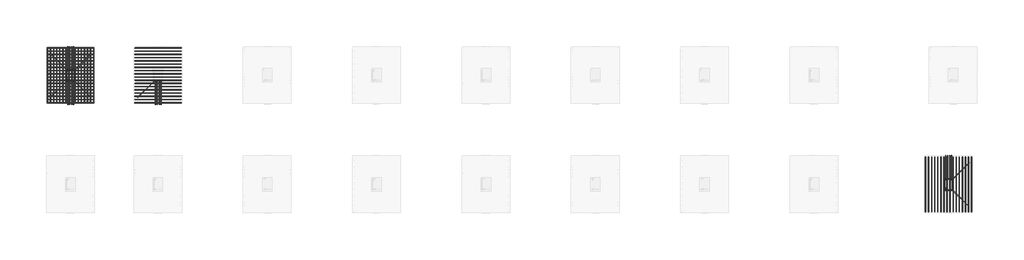
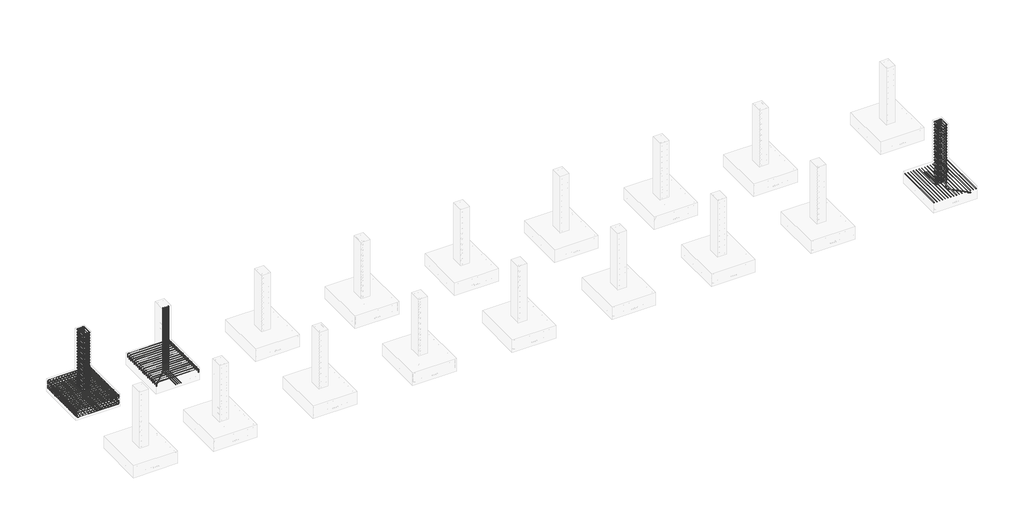
# One storey, part 13 of 33: 19 reinforcing bars.
"""IFC4 building model written with IfcOpenShell, lengths in millimetres."""

from ifc_helpers import new_model, si_unit, point, frame, origin, place, context, project, spatial, polyline, circle_curve, trimmed, segment, composite_curve, source, transform, mapped, element, save
from ifc_brep_helpers import swept_disk

model = new_model("IFC4")

# Units and contexts
model_context = context("Model", 3, world=origin())
ifc_project = project(units=[si_unit("LENGTHUNIT", "METRE", prefix="MILLI")], contexts=[model_context])

# Site, building, storey
site = spatial("IfcSite", under=ifc_project)
building = spatial("IfcBuilding", under=site)
storey = spatial("IfcBuildingStorey", under=building, Elevation=-3000.0)

# Reinforcing bars
placement = place(None, origin())
reinforcing_bar_shape = source(origin(), model_context, "Body", "SolidModel", [
    swept_disk(composite_curve([segment(polyline([(25452.7737106, -4557.7108134, -3122.7084113), (25452.7737106, -2037.7108134, -3122.7084113)]), True, "CONTINUOUS")], self_intersect=False), 6.35),
])
element("IfcReinforcingBar", 1, at=placement, inside=storey, context=model_context, shape_type="MappedRepresentation", body=[
    mapped(reinforcing_bar_shape, transform((0.0, 0.0, 0.0), x_axis=(1.0, 0.0, 0.0), y_axis=(0.0, 1.0, 0.0), z_axis=(0.0, 0.0, 1.0))),
    mapped(reinforcing_bar_shape, transform((140.4866667, 0.0, 0.0), x_axis=(1.0, 0.0, 0.0), y_axis=(0.0, 1.0, 0.0), z_axis=(0.0, 0.0, 1.0))),
    mapped(reinforcing_bar_shape, transform((280.9733333, 0.0, 0.0), x_axis=(1.0, 0.0, 0.0), y_axis=(0.0, 1.0, 0.0), z_axis=(0.0, 0.0, 1.0))),
    mapped(reinforcing_bar_shape, transform((421.46, 0.0, 0.0), x_axis=(1.0, 0.0, 0.0), y_axis=(0.0, 1.0, 0.0), z_axis=(0.0, 0.0, 1.0))),
    mapped(reinforcing_bar_shape, transform((561.9466667, 0.0, 0.0), x_axis=(1.0, 0.0, 0.0), y_axis=(0.0, 1.0, 0.0), z_axis=(0.0, 0.0, 1.0))),
    mapped(reinforcing_bar_shape, transform((702.4333333, 0.0, 0.0), x_axis=(1.0, 0.0, 0.0), y_axis=(0.0, 1.0, 0.0), z_axis=(0.0, 0.0, 1.0))),
    mapped(reinforcing_bar_shape, transform((842.92, 0.0, 0.0), x_axis=(1.0, 0.0, 0.0), y_axis=(0.0, 1.0, 0.0), z_axis=(0.0, 0.0, 1.0))),
    mapped(reinforcing_bar_shape, transform((983.4066667, 0.0, 0.0), x_axis=(1.0, 0.0, 0.0), y_axis=(0.0, 1.0, 0.0), z_axis=(0.0, 0.0, 1.0))),
    mapped(reinforcing_bar_shape, transform((1123.8933333, 0.0, 0.0), x_axis=(1.0, 0.0, 0.0), y_axis=(0.0, 1.0, 0.0), z_axis=(0.0, 0.0, 1.0))),
    mapped(reinforcing_bar_shape, transform((1264.38, 0.0, 0.0), x_axis=(1.0, 0.0, 0.0), y_axis=(0.0, 1.0, 0.0), z_axis=(0.0, 0.0, 1.0))),
    mapped(reinforcing_bar_shape, transform((1404.8666667, 0.0, 0.0), x_axis=(1.0, 0.0, 0.0), y_axis=(0.0, 1.0, 0.0), z_axis=(0.0, 0.0, 1.0))),
    mapped(reinforcing_bar_shape, transform((1545.3533333, 0.0, 0.0), x_axis=(1.0, 0.0, 0.0), y_axis=(0.0, 1.0, 0.0), z_axis=(0.0, 0.0, 1.0))),
    mapped(reinforcing_bar_shape, transform((1685.84, 0.0, 0.0), x_axis=(1.0, 0.0, 0.0), y_axis=(0.0, 1.0, 0.0), z_axis=(0.0, 0.0, 1.0))),
    mapped(reinforcing_bar_shape, transform((1826.3266667, 0.0, 0.0), x_axis=(1.0, 0.0, 0.0), y_axis=(0.0, 1.0, 0.0), z_axis=(0.0, 0.0, 1.0))),
    mapped(reinforcing_bar_shape, transform((1966.8133333, 0.0, 0.0), x_axis=(1.0, 0.0, 0.0), y_axis=(0.0, 1.0, 0.0), z_axis=(0.0, 0.0, 1.0))),
    mapped(reinforcing_bar_shape, transform((2107.3, 0.0, 0.0), x_axis=(1.0, 0.0, 0.0), y_axis=(0.0, 1.0, 0.0), z_axis=(0.0, 0.0, 1.0))),
])
reinforcing_bar_2_shape = source(origin(), model_context, "Body", "SolidModel", [
    swept_disk(composite_curve([segment(polyline([(-10693.4642742, 2955.9391866, -3240.0), (-10693.4642742, 2955.9391866, -3092.7)]), True, "CONTINUOUS"), segment(trimmed(circle_curve(frame((-10647.1142742, 2955.9391866, -3092.7), z_axis=(0.0, 1.0, 0.0), x_axis=(-46.350000000000364, 0.0, 0.0)), 46.35), [point((-10693.4642742, 2955.9391866, -3092.7))], [point((-10647.1142742, 2955.9391866, -3046.35))], True, "CARTESIAN"), True, "CONTINUOUS"), segment(polyline([(-10647.1142742, 2955.9391866, -3046.35), (-8632.5142742, 2955.9391866, -3046.35)]), True, "CONTINUOUS"), segment(trimmed(circle_curve(frame((-8632.5142742, 2955.9391866, -3092.7), z_axis=(0.0, 1.0, 0.0), x_axis=(0.0, 0.0, 46.34999999999991)), 46.35), [point((-8632.5142742, 2955.9391866, -3046.35))], [point((-8586.1642742, 2955.9391866, -3092.7))], True, "CARTESIAN"), True, "CONTINUOUS"), segment(polyline([(-8586.1642742, 2955.9391866, -3092.7), (-8586.1642742, 2955.9391866, -3240.0)]), True, "CONTINUOUS")], self_intersect=False), 6.35),
])
element("IfcReinforcingBar", 2, at=placement, inside=storey, context=model_context, shape_type="MappedRepresentation", body=[
    mapped(reinforcing_bar_2_shape, transform((0.0, 0.0, 0.0), x_axis=(1.0, 0.0, 0.0), y_axis=(0.0, 1.0, 0.0), z_axis=(0.0, 0.0, 1.0))),
    mapped(reinforcing_bar_2_shape, transform((0.0, -147.4882353, 0.0), x_axis=(1.0, 0.0, 0.0), y_axis=(0.0, 1.0, 0.0), z_axis=(0.0, 0.0, 1.0))),
    mapped(reinforcing_bar_2_shape, transform((0.0, -294.9764706, 0.0), x_axis=(1.0, 0.0, 0.0), y_axis=(0.0, 1.0, 0.0), z_axis=(0.0, 0.0, 1.0))),
    mapped(reinforcing_bar_2_shape, transform((0.0, -442.4647059, 0.0), x_axis=(1.0, 0.0, 0.0), y_axis=(0.0, 1.0, 0.0), z_axis=(0.0, 0.0, 1.0))),
    mapped(reinforcing_bar_2_shape, transform((0.0, -589.9529412, 0.0), x_axis=(1.0, 0.0, 0.0), y_axis=(0.0, 1.0, 0.0), z_axis=(0.0, 0.0, 1.0))),
    mapped(reinforcing_bar_2_shape, transform((0.0, -737.4411765, 0.0), x_axis=(1.0, 0.0, 0.0), y_axis=(0.0, 1.0, 0.0), z_axis=(0.0, 0.0, 1.0))),
    mapped(reinforcing_bar_2_shape, transform((0.0, -884.9294118, 0.0), x_axis=(1.0, 0.0, 0.0), y_axis=(0.0, 1.0, 0.0), z_axis=(0.0, 0.0, 1.0))),
    mapped(reinforcing_bar_2_shape, transform((0.0, -1032.4176471, 0.0), x_axis=(1.0, 0.0, 0.0), y_axis=(0.0, 1.0, 0.0), z_axis=(0.0, 0.0, 1.0))),
    mapped(reinforcing_bar_2_shape, transform((0.0, -1179.9058824, 0.0), x_axis=(1.0, 0.0, 0.0), y_axis=(0.0, 1.0, 0.0), z_axis=(0.0, 0.0, 1.0))),
    mapped(reinforcing_bar_2_shape, transform((0.0, -1327.3941176, 0.0), x_axis=(1.0, 0.0, 0.0), y_axis=(0.0, 1.0, 0.0), z_axis=(0.0, 0.0, 1.0))),
    mapped(reinforcing_bar_2_shape, transform((0.0, -1474.8823529, 0.0), x_axis=(1.0, 0.0, 0.0), y_axis=(0.0, 1.0, 0.0), z_axis=(0.0, 0.0, 1.0))),
    mapped(reinforcing_bar_2_shape, transform((0.0, -1622.3705882, 0.0), x_axis=(1.0, 0.0, 0.0), y_axis=(0.0, 1.0, 0.0), z_axis=(0.0, 0.0, 1.0))),
    mapped(reinforcing_bar_2_shape, transform((0.0, -1769.8588235, 0.0), x_axis=(1.0, 0.0, 0.0), y_axis=(0.0, 1.0, 0.0), z_axis=(0.0, 0.0, 1.0))),
    mapped(reinforcing_bar_2_shape, transform((0.0, -1917.3470588, 0.0), x_axis=(1.0, 0.0, 0.0), y_axis=(0.0, 1.0, 0.0), z_axis=(0.0, 0.0, 1.0))),
    mapped(reinforcing_bar_2_shape, transform((0.0, -2064.8352941, 0.0), x_axis=(1.0, 0.0, 0.0), y_axis=(0.0, 1.0, 0.0), z_axis=(0.0, 0.0, 1.0))),
    mapped(reinforcing_bar_2_shape, transform((0.0, -2212.3235294, 0.0), x_axis=(1.0, 0.0, 0.0), y_axis=(0.0, 1.0, 0.0), z_axis=(0.0, 0.0, 1.0))),
    mapped(reinforcing_bar_2_shape, transform((0.0, -2359.8117647, 0.0), x_axis=(1.0, 0.0, 0.0), y_axis=(0.0, 1.0, 0.0), z_axis=(0.0, 0.0, 1.0))),
    mapped(reinforcing_bar_2_shape, transform((0.0, -2507.3, 0.0), x_axis=(1.0, 0.0, 0.0), y_axis=(0.0, 1.0, 0.0), z_axis=(0.0, 0.0, 1.0))),
])
reinforcing_bar_3_shape = source(origin(), model_context, "Body", "SolidModel", [
    swept_disk(composite_curve([segment(polyline([(-14693.4642742, 2955.9391866, -3240.0), (-14693.4642742, 2955.9391866, -3092.7)]), True, "CONTINUOUS"), segment(trimmed(circle_curve(frame((-14647.1142742, 2955.9391866, -3092.7), z_axis=(0.0, 1.0, 0.0), x_axis=(-46.350000000000364, 0.0, 0.0)), 46.35), [point((-14693.4642742, 2955.9391866, -3092.7))], [point((-14647.1142742, 2955.9391866, -3046.35))], True, "CARTESIAN"), True, "CONTINUOUS"), segment(polyline([(-14647.1142742, 2955.9391866, -3046.35), (-12632.5142742, 2955.9391866, -3046.35)]), True, "CONTINUOUS"), segment(trimmed(circle_curve(frame((-12632.5142742, 2955.9391866, -3092.7), z_axis=(0.0, 1.0, 0.0), x_axis=(0.0, 0.0, 46.34999999999991)), 46.35), [point((-12632.5142742, 2955.9391866, -3046.35))], [point((-12586.1642742, 2955.9391866, -3092.7))], True, "CARTESIAN"), True, "CONTINUOUS"), segment(polyline([(-12586.1642742, 2955.9391866, -3092.7), (-12586.1642742, 2955.9391866, -3240.0)]), True, "CONTINUOUS")], self_intersect=False), 6.35),
])
element("IfcReinforcingBar", 3, at=placement, inside=storey, context=model_context, shape_type="MappedRepresentation", body=[
    mapped(reinforcing_bar_3_shape, transform((0.0, 0.0, 0.0), x_axis=(1.0, 0.0, 0.0), y_axis=(0.0, 1.0, 0.0), z_axis=(0.0, 0.0, 1.0))),
    mapped(reinforcing_bar_3_shape, transform((0.0, -147.4882353, 0.0), x_axis=(1.0, 0.0, 0.0), y_axis=(0.0, 1.0, 0.0), z_axis=(0.0, 0.0, 1.0))),
    mapped(reinforcing_bar_3_shape, transform((0.0, -294.9764706, 0.0), x_axis=(1.0, 0.0, 0.0), y_axis=(0.0, 1.0, 0.0), z_axis=(0.0, 0.0, 1.0))),
    mapped(reinforcing_bar_3_shape, transform((0.0, -442.4647059, 0.0), x_axis=(1.0, 0.0, 0.0), y_axis=(0.0, 1.0, 0.0), z_axis=(0.0, 0.0, 1.0))),
    mapped(reinforcing_bar_3_shape, transform((0.0, -589.9529412, 0.0), x_axis=(1.0, 0.0, 0.0), y_axis=(0.0, 1.0, 0.0), z_axis=(0.0, 0.0, 1.0))),
    mapped(reinforcing_bar_3_shape, transform((0.0, -737.4411765, 0.0), x_axis=(1.0, 0.0, 0.0), y_axis=(0.0, 1.0, 0.0), z_axis=(0.0, 0.0, 1.0))),
    mapped(reinforcing_bar_3_shape, transform((0.0, -884.9294118, 0.0), x_axis=(1.0, 0.0, 0.0), y_axis=(0.0, 1.0, 0.0), z_axis=(0.0, 0.0, 1.0))),
    mapped(reinforcing_bar_3_shape, transform((0.0, -1032.4176471, 0.0), x_axis=(1.0, 0.0, 0.0), y_axis=(0.0, 1.0, 0.0), z_axis=(0.0, 0.0, 1.0))),
    mapped(reinforcing_bar_3_shape, transform((0.0, -1179.9058824, 0.0), x_axis=(1.0, 0.0, 0.0), y_axis=(0.0, 1.0, 0.0), z_axis=(0.0, 0.0, 1.0))),
    mapped(reinforcing_bar_3_shape, transform((0.0, -1327.3941176, 0.0), x_axis=(1.0, 0.0, 0.0), y_axis=(0.0, 1.0, 0.0), z_axis=(0.0, 0.0, 1.0))),
    mapped(reinforcing_bar_3_shape, transform((0.0, -1474.8823529, 0.0), x_axis=(1.0, 0.0, 0.0), y_axis=(0.0, 1.0, 0.0), z_axis=(0.0, 0.0, 1.0))),
    mapped(reinforcing_bar_3_shape, transform((0.0, -1622.3705882, 0.0), x_axis=(1.0, 0.0, 0.0), y_axis=(0.0, 1.0, 0.0), z_axis=(0.0, 0.0, 1.0))),
    mapped(reinforcing_bar_3_shape, transform((0.0, -1769.8588235, 0.0), x_axis=(1.0, 0.0, 0.0), y_axis=(0.0, 1.0, 0.0), z_axis=(0.0, 0.0, 1.0))),
    mapped(reinforcing_bar_3_shape, transform((0.0, -1917.3470588, 0.0), x_axis=(1.0, 0.0, 0.0), y_axis=(0.0, 1.0, 0.0), z_axis=(0.0, 0.0, 1.0))),
    mapped(reinforcing_bar_3_shape, transform((0.0, -2064.8352941, 0.0), x_axis=(1.0, 0.0, 0.0), y_axis=(0.0, 1.0, 0.0), z_axis=(0.0, 0.0, 1.0))),
    mapped(reinforcing_bar_3_shape, transform((0.0, -2212.3235294, 0.0), x_axis=(1.0, 0.0, 0.0), y_axis=(0.0, 1.0, 0.0), z_axis=(0.0, 0.0, 1.0))),
    mapped(reinforcing_bar_3_shape, transform((0.0, -2359.8117647, 0.0), x_axis=(1.0, 0.0, 0.0), y_axis=(0.0, 1.0, 0.0), z_axis=(0.0, 0.0, 1.0))),
    mapped(reinforcing_bar_3_shape, transform((0.0, -2507.3, 0.0), x_axis=(1.0, 0.0, 0.0), y_axis=(0.0, 1.0, 0.0), z_axis=(0.0, 0.0, 1.0))),
])
reinforcing_bar_4_shape = source(origin(), model_context, "Body", "SolidModel", [
    swept_disk(composite_curve([segment(polyline([(-12586.1642742, 2955.9391866, -3330.080452), (-12586.1642742, 2955.9391866, -3477.380452)]), True, "CONTINUOUS"), segment(trimmed(circle_curve(frame((-12632.5142742, 2955.9391866, -3477.380452), z_axis=(0.0, 1.0, 0.0), x_axis=(46.350000000000364, 0.0, 0.0)), 46.35), [point((-12586.1642742, 2955.9391866, -3477.380452))], [point((-12632.5142742, 2955.9391866, -3523.730452))], True, "CARTESIAN"), True, "CONTINUOUS"), segment(polyline([(-12632.5142742, 2955.9391866, -3523.730452), (-14647.1142742, 2955.9391866, -3523.730452)]), True, "CONTINUOUS"), segment(trimmed(circle_curve(frame((-14647.1142742, 2955.9391866, -3477.380452), z_axis=(0.0, 1.0, 0.0), x_axis=(0.0, 0.0, -46.34999999999991)), 46.35), [point((-14647.1142742, 2955.9391866, -3523.730452))], [point((-14693.4642742, 2955.9391866, -3477.380452))], True, "CARTESIAN"), True, "CONTINUOUS"), segment(polyline([(-14693.4642742, 2955.9391866, -3477.380452), (-14693.4642742, 2955.9391866, -3330.080452)]), True, "CONTINUOUS")], self_intersect=False), 6.35),
])
element("IfcReinforcingBar", 4, at=placement, inside=storey, context=model_context, shape_type="MappedRepresentation", body=[
    mapped(reinforcing_bar_4_shape, transform((0.0, 0.0, 0.0), x_axis=(1.0, 0.0, 0.0), y_axis=(0.0, 1.0, 0.0), z_axis=(0.0, 0.0, 1.0))),
    mapped(reinforcing_bar_4_shape, transform((0.0, -147.4882353, 0.0), x_axis=(1.0, 0.0, 0.0), y_axis=(0.0, 1.0, 0.0), z_axis=(0.0, 0.0, 1.0))),
    mapped(reinforcing_bar_4_shape, transform((0.0, -294.9764706, 0.0), x_axis=(1.0, 0.0, 0.0), y_axis=(0.0, 1.0, 0.0), z_axis=(0.0, 0.0, 1.0))),
    mapped(reinforcing_bar_4_shape, transform((0.0, -442.4647059, 0.0), x_axis=(1.0, 0.0, 0.0), y_axis=(0.0, 1.0, 0.0), z_axis=(0.0, 0.0, 1.0))),
    mapped(reinforcing_bar_4_shape, transform((0.0, -589.9529412, 0.0), x_axis=(1.0, 0.0, 0.0), y_axis=(0.0, 1.0, 0.0), z_axis=(0.0, 0.0, 1.0))),
    mapped(reinforcing_bar_4_shape, transform((0.0, -737.4411765, 0.0), x_axis=(1.0, 0.0, 0.0), y_axis=(0.0, 1.0, 0.0), z_axis=(0.0, 0.0, 1.0))),
    mapped(reinforcing_bar_4_shape, transform((0.0, -884.9294118, 0.0), x_axis=(1.0, 0.0, 0.0), y_axis=(0.0, 1.0, 0.0), z_axis=(0.0, 0.0, 1.0))),
    mapped(reinforcing_bar_4_shape, transform((0.0, -1032.4176471, 0.0), x_axis=(1.0, 0.0, 0.0), y_axis=(0.0, 1.0, 0.0), z_axis=(0.0, 0.0, 1.0))),
    mapped(reinforcing_bar_4_shape, transform((0.0, -1179.9058824, 0.0), x_axis=(1.0, 0.0, 0.0), y_axis=(0.0, 1.0, 0.0), z_axis=(0.0, 0.0, 1.0))),
    mapped(reinforcing_bar_4_shape, transform((0.0, -1327.3941176, 0.0), x_axis=(1.0, 0.0, 0.0), y_axis=(0.0, 1.0, 0.0), z_axis=(0.0, 0.0, 1.0))),
    mapped(reinforcing_bar_4_shape, transform((0.0, -1474.8823529, 0.0), x_axis=(1.0, 0.0, 0.0), y_axis=(0.0, 1.0, 0.0), z_axis=(0.0, 0.0, 1.0))),
    mapped(reinforcing_bar_4_shape, transform((0.0, -1622.3705882, 0.0), x_axis=(1.0, 0.0, 0.0), y_axis=(0.0, 1.0, 0.0), z_axis=(0.0, 0.0, 1.0))),
    mapped(reinforcing_bar_4_shape, transform((0.0, -1769.8588235, 0.0), x_axis=(1.0, 0.0, 0.0), y_axis=(0.0, 1.0, 0.0), z_axis=(0.0, 0.0, 1.0))),
    mapped(reinforcing_bar_4_shape, transform((0.0, -1917.3470588, 0.0), x_axis=(1.0, 0.0, 0.0), y_axis=(0.0, 1.0, 0.0), z_axis=(0.0, 0.0, 1.0))),
    mapped(reinforcing_bar_4_shape, transform((0.0, -2064.8352941, 0.0), x_axis=(1.0, 0.0, 0.0), y_axis=(0.0, 1.0, 0.0), z_axis=(0.0, 0.0, 1.0))),
    mapped(reinforcing_bar_4_shape, transform((0.0, -2212.3235294, 0.0), x_axis=(1.0, 0.0, 0.0), y_axis=(0.0, 1.0, 0.0), z_axis=(0.0, 0.0, 1.0))),
    mapped(reinforcing_bar_4_shape, transform((0.0, -2359.8117647, 0.0), x_axis=(1.0, 0.0, 0.0), y_axis=(0.0, 1.0, 0.0), z_axis=(0.0, 0.0, 1.0))),
    mapped(reinforcing_bar_4_shape, transform((0.0, -2507.3, 0.0), x_axis=(1.0, 0.0, 0.0), y_axis=(0.0, 1.0, 0.0), z_axis=(0.0, 0.0, 1.0))),
])
reinforcing_bar_5_shape = source(origin(), model_context, "Body", "SolidModel", [
    swept_disk(composite_curve([segment(polyline([(-12586.1642742, 442.2891866, -3447.8614173), (-12586.1642742, 2962.2891866, -3447.8614173)]), True, "CONTINUOUS")], self_intersect=False), 6.35),
])
element("IfcReinforcingBar", 5, at=placement, inside=storey, context=model_context, shape_type="MappedRepresentation", body=[
    mapped(reinforcing_bar_5_shape, transform((0.0, 0.0, 0.0), x_axis=(1.0, 0.0, 0.0), y_axis=(0.0, 1.0, 0.0), z_axis=(0.0, 0.0, 1.0))),
    mapped(reinforcing_bar_5_shape, transform((-140.4866667, 0.0, 0.0), x_axis=(1.0, 0.0, 0.0), y_axis=(0.0, 1.0, 0.0), z_axis=(0.0, 0.0, 1.0))),
    mapped(reinforcing_bar_5_shape, transform((-280.9733333, 0.0, 0.0), x_axis=(1.0, 0.0, 0.0), y_axis=(0.0, 1.0, 0.0), z_axis=(0.0, 0.0, 1.0))),
    mapped(reinforcing_bar_5_shape, transform((-421.46, 0.0, 0.0), x_axis=(1.0, 0.0, 0.0), y_axis=(0.0, 1.0, 0.0), z_axis=(0.0, 0.0, 1.0))),
    mapped(reinforcing_bar_5_shape, transform((-561.9466667, 0.0, 0.0), x_axis=(1.0, 0.0, 0.0), y_axis=(0.0, 1.0, 0.0), z_axis=(0.0, 0.0, 1.0))),
    mapped(reinforcing_bar_5_shape, transform((-702.4333333, 0.0, 0.0), x_axis=(1.0, 0.0, 0.0), y_axis=(0.0, 1.0, 0.0), z_axis=(0.0, 0.0, 1.0))),
    mapped(reinforcing_bar_5_shape, transform((-842.92, 0.0, 0.0), x_axis=(1.0, 0.0, 0.0), y_axis=(0.0, 1.0, 0.0), z_axis=(0.0, 0.0, 1.0))),
    mapped(reinforcing_bar_5_shape, transform((-983.4066667, 0.0, 0.0), x_axis=(1.0, 0.0, 0.0), y_axis=(0.0, 1.0, 0.0), z_axis=(0.0, 0.0, 1.0))),
    mapped(reinforcing_bar_5_shape, transform((-1123.8933333, 0.0, 0.0), x_axis=(1.0, 0.0, 0.0), y_axis=(0.0, 1.0, 0.0), z_axis=(0.0, 0.0, 1.0))),
    mapped(reinforcing_bar_5_shape, transform((-1264.38, 0.0, 0.0), x_axis=(1.0, 0.0, 0.0), y_axis=(0.0, 1.0, 0.0), z_axis=(0.0, 0.0, 1.0))),
    mapped(reinforcing_bar_5_shape, transform((-1404.8666667, 0.0, 0.0), x_axis=(1.0, 0.0, 0.0), y_axis=(0.0, 1.0, 0.0), z_axis=(0.0, 0.0, 1.0))),
    mapped(reinforcing_bar_5_shape, transform((-1545.3533333, 0.0, 0.0), x_axis=(1.0, 0.0, 0.0), y_axis=(0.0, 1.0, 0.0), z_axis=(0.0, 0.0, 1.0))),
    mapped(reinforcing_bar_5_shape, transform((-1685.84, 0.0, 0.0), x_axis=(1.0, 0.0, 0.0), y_axis=(0.0, 1.0, 0.0), z_axis=(0.0, 0.0, 1.0))),
    mapped(reinforcing_bar_5_shape, transform((-1826.3266667, 0.0, 0.0), x_axis=(1.0, 0.0, 0.0), y_axis=(0.0, 1.0, 0.0), z_axis=(0.0, 0.0, 1.0))),
    mapped(reinforcing_bar_5_shape, transform((-1966.8133333, 0.0, 0.0), x_axis=(1.0, 0.0, 0.0), y_axis=(0.0, 1.0, 0.0), z_axis=(0.0, 0.0, 1.0))),
    mapped(reinforcing_bar_5_shape, transform((-2107.3, 0.0, 0.0), x_axis=(1.0, 0.0, 0.0), y_axis=(0.0, 1.0, 0.0), z_axis=(0.0, 0.0, 1.0))),
])
reinforcing_bar_6_shape = source(origin(), model_context, "Body", "SolidModel", [
    swept_disk(composite_curve([segment(polyline([(-14693.4642742, 442.2891866, -3122.7084113), (-14693.4642742, 2962.2891866, -3122.7084113)]), True, "CONTINUOUS")], self_intersect=False), 6.35),
])
element("IfcReinforcingBar", 6, at=placement, inside=storey, context=model_context, shape_type="MappedRepresentation", body=[
    mapped(reinforcing_bar_6_shape, transform((0.0, 0.0, 0.0), x_axis=(1.0, 0.0, 0.0), y_axis=(0.0, 1.0, 0.0), z_axis=(0.0, 0.0, 1.0))),
    mapped(reinforcing_bar_6_shape, transform((140.4866667, 0.0, 0.0), x_axis=(1.0, 0.0, 0.0), y_axis=(0.0, 1.0, 0.0), z_axis=(0.0, 0.0, 1.0))),
    mapped(reinforcing_bar_6_shape, transform((280.9733333, 0.0, 0.0), x_axis=(1.0, 0.0, 0.0), y_axis=(0.0, 1.0, 0.0), z_axis=(0.0, 0.0, 1.0))),
    mapped(reinforcing_bar_6_shape, transform((421.46, 0.0, 0.0), x_axis=(1.0, 0.0, 0.0), y_axis=(0.0, 1.0, 0.0), z_axis=(0.0, 0.0, 1.0))),
    mapped(reinforcing_bar_6_shape, transform((561.9466667, 0.0, 0.0), x_axis=(1.0, 0.0, 0.0), y_axis=(0.0, 1.0, 0.0), z_axis=(0.0, 0.0, 1.0))),
    mapped(reinforcing_bar_6_shape, transform((702.4333333, 0.0, 0.0), x_axis=(1.0, 0.0, 0.0), y_axis=(0.0, 1.0, 0.0), z_axis=(0.0, 0.0, 1.0))),
    mapped(reinforcing_bar_6_shape, transform((842.92, 0.0, 0.0), x_axis=(1.0, 0.0, 0.0), y_axis=(0.0, 1.0, 0.0), z_axis=(0.0, 0.0, 1.0))),
    mapped(reinforcing_bar_6_shape, transform((983.4066667, 0.0, 0.0), x_axis=(1.0, 0.0, 0.0), y_axis=(0.0, 1.0, 0.0), z_axis=(0.0, 0.0, 1.0))),
    mapped(reinforcing_bar_6_shape, transform((1123.8933333, 0.0, 0.0), x_axis=(1.0, 0.0, 0.0), y_axis=(0.0, 1.0, 0.0), z_axis=(0.0, 0.0, 1.0))),
    mapped(reinforcing_bar_6_shape, transform((1264.38, 0.0, 0.0), x_axis=(1.0, 0.0, 0.0), y_axis=(0.0, 1.0, 0.0), z_axis=(0.0, 0.0, 1.0))),
    mapped(reinforcing_bar_6_shape, transform((1404.8666667, 0.0, 0.0), x_axis=(1.0, 0.0, 0.0), y_axis=(0.0, 1.0, 0.0), z_axis=(0.0, 0.0, 1.0))),
    mapped(reinforcing_bar_6_shape, transform((1545.3533333, 0.0, 0.0), x_axis=(1.0, 0.0, 0.0), y_axis=(0.0, 1.0, 0.0), z_axis=(0.0, 0.0, 1.0))),
    mapped(reinforcing_bar_6_shape, transform((1685.84, 0.0, 0.0), x_axis=(1.0, 0.0, 0.0), y_axis=(0.0, 1.0, 0.0), z_axis=(0.0, 0.0, 1.0))),
    mapped(reinforcing_bar_6_shape, transform((1826.3266667, 0.0, 0.0), x_axis=(1.0, 0.0, 0.0), y_axis=(0.0, 1.0, 0.0), z_axis=(0.0, 0.0, 1.0))),
    mapped(reinforcing_bar_6_shape, transform((1966.8133333, 0.0, 0.0), x_axis=(1.0, 0.0, 0.0), y_axis=(0.0, 1.0, 0.0), z_axis=(0.0, 0.0, 1.0))),
    mapped(reinforcing_bar_6_shape, transform((2107.3, 0.0, 0.0), x_axis=(1.0, 0.0, 0.0), y_axis=(0.0, 1.0, 0.0), z_axis=(0.0, 0.0, 1.0))),
])
reinforcing_bar_7_shape = source(origin(), model_context, "Body", "SolidModel", [
    swept_disk(composite_curve([segment(polyline([(-13753.5385089, 1553.1005472, -2953.65), (-13809.2820718, 1497.3569842, -2953.65)]), True, "CONTINUOUS"), segment(trimmed(circle_curve(frame((-13787.1142742, 1475.1891866, -2953.65), z_axis=(0.0, 0.0, 1.0), x_axis=(-22.167797600000995, 22.167797599999858, 0.0)), 31.35), [point((-13809.2820718, 1497.3569842, -2953.65))], [point((-13787.1142742, 1443.8391866, -2953.65))], True, "CARTESIAN"), True, "CONTINUOUS"), segment(polyline([(-13787.1142742, 1443.8391866, -2953.65), (-13492.5142742, 1443.8391866, -2953.65)]), True, "CONTINUOUS"), segment(trimmed(circle_curve(frame((-13492.5142742, 1475.1891866, -2953.65), z_axis=(0.0, 0.0, 1.0), x_axis=(0.0, -31.350000000000136, 0.0)), 31.35), [point((-13492.5142742, 1443.8391866, -2953.65))], [point((-13461.1642742, 1475.1891866, -2953.65))], True, "CARTESIAN"), True, "CONTINUOUS"), segment(polyline([(-13461.1642742, 1475.1891866, -2953.65), (-13461.1642742, 1929.3891866, -2953.65)]), True, "CONTINUOUS"), segment(trimmed(circle_curve(frame((-13492.4944891, 1929.3891866, -2954.7636125), z_axis=(-0.0355219283344822, 0.0, 0.9993688971583016), x_axis=(31.33021489999919, 0.0, 1.1136124999998174)), 31.35), [point((-13461.1642742, 1929.3891866, -2953.65))], [point((-13492.4944891, 1960.7391866, -2954.7636125))], True, "CARTESIAN"), True, "CONTINUOUS"), segment(polyline([(-13492.4944891, 1960.7391866, -2954.7636125), (-13787.1340593, 1960.7391866, -2965.2363875)]), True, "CONTINUOUS"), segment(trimmed(circle_curve(frame((-13787.1340593, 1929.3891866, -2965.2363875), z_axis=(-0.0355219283344822, 0.0, 0.9993688971583016), x_axis=(0.0, 31.350000000000136, 0.0)), 31.35), [point((-13787.1340593, 1960.7391866, -2965.2363875))], [point((-13818.4642742, 1929.3891866, -2966.35))], True, "CARTESIAN"), True, "CONTINUOUS"), segment(polyline([(-13818.4642742, 1929.3891866, -2966.35), (-13818.4642742, 1475.1891866, -2966.35)]), True, "CONTINUOUS"), segment(trimmed(circle_curve(frame((-13787.1142742, 1475.1891866, -2966.35), z_axis=(0.0, 0.0, 1.0), x_axis=(-31.350000000000364, 0.0, 0.0)), 31.35), [point((-13818.4642742, 1475.1891866, -2966.35))], [point((-13764.9464766, 1453.021389, -2966.35))], True, "CARTESIAN"), True, "CONTINUOUS"), segment(polyline([(-13764.9464766, 1453.021389, -2966.35), (-13709.2029137, 1508.764952, -2966.35)]), True, "CONTINUOUS")], self_intersect=False), 6.35),
])
element("IfcReinforcingBar", 7, at=placement, inside=storey, context=model_context, shape_type="MappedRepresentation", body=[
    mapped(reinforcing_bar_7_shape, transform((0.0, 0.0, 0.0), x_axis=(1.0, 0.0, 0.0), y_axis=(0.0, 1.0, 0.0), z_axis=(0.0, 0.0, 1.0))),
    mapped(reinforcing_bar_7_shape, transform((0.0, 0.0, 145.365), x_axis=(1.0, 0.0, 0.0), y_axis=(0.0, 1.0, 0.0), z_axis=(0.0, 0.0, 1.0))),
    mapped(reinforcing_bar_7_shape, transform((0.0, 0.0, 290.73), x_axis=(1.0, 0.0, 0.0), y_axis=(0.0, 1.0, 0.0), z_axis=(0.0, 0.0, 1.0))),
    mapped(reinforcing_bar_7_shape, transform((0.0, 0.0, 436.095), x_axis=(1.0, 0.0, 0.0), y_axis=(0.0, 1.0, 0.0), z_axis=(0.0, 0.0, 1.0))),
    mapped(reinforcing_bar_7_shape, transform((0.0, 0.0, 581.46), x_axis=(1.0, 0.0, 0.0), y_axis=(0.0, 1.0, 0.0), z_axis=(0.0, 0.0, 1.0))),
    mapped(reinforcing_bar_7_shape, transform((0.0, 0.0, 726.825), x_axis=(1.0, 0.0, 0.0), y_axis=(0.0, 1.0, 0.0), z_axis=(0.0, 0.0, 1.0))),
    mapped(reinforcing_bar_7_shape, transform((0.0, 0.0, 872.19), x_axis=(1.0, 0.0, 0.0), y_axis=(0.0, 1.0, 0.0), z_axis=(0.0, 0.0, 1.0))),
    mapped(reinforcing_bar_7_shape, transform((0.0, 0.0, 1017.555), x_axis=(1.0, 0.0, 0.0), y_axis=(0.0, 1.0, 0.0), z_axis=(0.0, 0.0, 1.0))),
    mapped(reinforcing_bar_7_shape, transform((0.0, 0.0, 1162.92), x_axis=(1.0, 0.0, 0.0), y_axis=(0.0, 1.0, 0.0), z_axis=(0.0, 0.0, 1.0))),
    mapped(reinforcing_bar_7_shape, transform((0.0, 0.0, 1308.285), x_axis=(1.0, 0.0, 0.0), y_axis=(0.0, 1.0, 0.0), z_axis=(0.0, 0.0, 1.0))),
    mapped(reinforcing_bar_7_shape, transform((0.0, 0.0, 1453.65), x_axis=(1.0, 0.0, 0.0), y_axis=(0.0, 1.0, 0.0), z_axis=(0.0, 0.0, 1.0))),
    mapped(reinforcing_bar_7_shape, transform((0.0, 0.0, 1599.015), x_axis=(1.0, 0.0, 0.0), y_axis=(0.0, 1.0, 0.0), z_axis=(0.0, 0.0, 1.0))),
    mapped(reinforcing_bar_7_shape, transform((0.0, 0.0, 1744.38), x_axis=(1.0, 0.0, 0.0), y_axis=(0.0, 1.0, 0.0), z_axis=(0.0, 0.0, 1.0))),
    mapped(reinforcing_bar_7_shape, transform((0.0, 0.0, 1889.745), x_axis=(1.0, 0.0, 0.0), y_axis=(0.0, 1.0, 0.0), z_axis=(0.0, 0.0, 1.0))),
    mapped(reinforcing_bar_7_shape, transform((0.0, 0.0, 2035.11), x_axis=(1.0, 0.0, 0.0), y_axis=(0.0, 1.0, 0.0), z_axis=(0.0, 0.0, 1.0))),
    mapped(reinforcing_bar_7_shape, transform((0.0, 0.0, 2180.475), x_axis=(1.0, 0.0, 0.0), y_axis=(0.0, 1.0, 0.0), z_axis=(0.0, 0.0, 1.0))),
    mapped(reinforcing_bar_7_shape, transform((0.0, 0.0, 2325.84), x_axis=(1.0, 0.0, 0.0), y_axis=(0.0, 1.0, 0.0), z_axis=(0.0, 0.0, 1.0))),
    mapped(reinforcing_bar_7_shape, transform((0.0, 0.0, 2471.205), x_axis=(1.0, 0.0, 0.0), y_axis=(0.0, 1.0, 0.0), z_axis=(0.0, 0.0, 1.0))),
    mapped(reinforcing_bar_7_shape, transform((0.0, 0.0, 2616.57), x_axis=(1.0, 0.0, 0.0), y_axis=(0.0, 1.0, 0.0), z_axis=(0.0, 0.0, 1.0))),
    mapped(reinforcing_bar_7_shape, transform((0.0, 0.0, 2761.935), x_axis=(1.0, 0.0, 0.0), y_axis=(0.0, 1.0, 0.0), z_axis=(0.0, 0.0, 1.0))),
    mapped(reinforcing_bar_7_shape, transform((0.0, 0.0, 2907.3), x_axis=(1.0, 0.0, 0.0), y_axis=(0.0, 1.0, 0.0), z_axis=(0.0, 0.0, 1.0))),
])
element("IfcReinforcingBar", 8, at=placement, inside=storey, context=model_context, shape_type="SolidModel", body=[
    swept_disk(composite_curve([segment(polyline([(-13786.7956786, 1478.3660586, -40.0), (-13786.7956786, 1478.3660586, -3393.65)]), True, "CONTINUOUS"), segment(trimmed(circle_curve(frame((-13819.5700779, 1445.5916593, -3393.65), z_axis=(-0.7071067811865446, 0.7071067811865505, 0.0), x_axis=(32.77439930000037, 32.77439930000014, 0.0)), 46.35), [point((-13786.7956786, 1478.3660586, -3393.65))], [point((-13819.5700779, 1445.5916593, -3440.0))], True, "CARTESIAN"), True, "CONTINUOUS"), segment(polyline([(-13819.5700779, 1445.5916593, -3440.0), (-14564.6131379, 700.5485993, -3440.0)]), True, "CONTINUOUS")], self_intersect=False), 6.35),
])
element("IfcReinforcingBar", 9, at=placement, inside=storey, context=model_context, shape_type="SolidModel", body=[
    swept_disk(composite_curve([segment(polyline([(-13768.8975726, 1908.3142087, -40.0), (-13768.8975726, 1908.3142087, -3361.434517)]), True, "CONTINUOUS"), segment(trimmed(circle_curve(frame((-13801.6719719, 1941.088608, -3361.434517), z_axis=(0.7071067811865539, 0.7071067811865411, 0.0), x_axis=(32.77439929999855, -32.774399299999914, 0.0)), 46.35), [point((-13768.8975726, 1908.3142087, -3361.434517))], [point((-13801.6719719, 1941.088608, -3407.784517))], True, "CARTESIAN"), True, "CONTINUOUS"), segment(polyline([(-13801.6719719, 1941.088608, -3407.784517), (-14564.6131379, 2704.029774, -3407.784517)]), True, "CONTINUOUS")], self_intersect=False), 6.35),
])
element("IfcReinforcingBar", 10, at=placement, inside=storey, context=model_context, shape_type="SolidModel", body=[
    swept_disk(composite_curve([segment(polyline([(-13492.8328699, 1478.3660586, -40.0), (-13492.8328699, 1478.3660586, -3393.65)]), True, "CONTINUOUS"), segment(trimmed(circle_curve(frame((-13460.0584706, 1445.5916593, -3393.65), z_axis=(-0.7071067811865493, -0.7071067811865459, 0.0), x_axis=(-32.77439929999855, 32.77439930000014, 0.0)), 46.35), [point((-13492.8328699, 1478.3660586, -3393.65))], [point((-13460.0584706, 1445.5916593, -3440.0))], True, "CARTESIAN"), True, "CONTINUOUS"), segment(polyline([(-13460.0584706, 1445.5916593, -3440.0), (-12715.0154106, 700.5485993, -3440.0)]), True, "CONTINUOUS")], self_intersect=False), 6.35),
])
element("IfcReinforcingBar", 11, at=placement, inside=storey, context=model_context, shape_type="SolidModel", body=[
    swept_disk(composite_curve([segment(polyline([(-13474.2315783, 1926.2123147, -30.2564663), (-13474.2315783, 1926.2123147, -3383.9064663)]), True, "CONTINUOUS"), segment(trimmed(circle_curve(frame((-13441.457179, 1958.986714, -3383.9064663), z_axis=(0.7071067811865493, -0.7071067811865459, 0.0), x_axis=(-32.77439929999855, -32.774399299999914, 0.0)), 46.35), [point((-13474.2315783, 1926.2123147, -3383.9064663))], [point((-13441.457179, 1958.986714, -3430.2564663))], True, "CARTESIAN"), True, "CONTINUOUS"), segment(polyline([(-13441.457179, 1958.986714, -3430.2564663), (-12696.414119, 2704.029774, -3430.2564663)]), True, "CONTINUOUS")], self_intersect=False), 6.35),
])
reinforcing_bar_8_shape = source(origin(), model_context, "Body", "SolidModel", [
    swept_disk(composite_curve([segment(polyline([(-13763.8841678, 1928.0721866, -40.0), (-13763.8841678, 1928.0721866, -3393.65)]), True, "CONTINUOUS"), segment(trimmed(circle_curve(frame((-13763.8841678, 1974.4221866, -3393.65), z_axis=(1.0, 0.0, 0.0), x_axis=(0.0, -46.350000000000136, 0.0)), 46.35), [point((-13763.8841678, 1928.0721866, -3393.65))], [point((-13763.8841678, 1974.4221866, -3440.0))], True, "CARTESIAN"), True, "CONTINUOUS"), segment(polyline([(-13763.8841678, 1974.4221866, -3440.0), (-13763.8841678, 3028.0721866, -3440.0)]), True, "CONTINUOUS")], self_intersect=False), 6.35),
])
element("IfcReinforcingBar", 12, at=placement, inside=storey, context=model_context, shape_type="MappedRepresentation", body=[
    mapped(reinforcing_bar_8_shape, transform((0.0, 0.0, 0.0), x_axis=(1.0, 0.0, 0.0), y_axis=(0.0, 1.0, 0.0), z_axis=(0.0, 0.0, 1.0))),
    mapped(reinforcing_bar_8_shape, transform((86.8979716, 0.0, 0.0), x_axis=(1.0, 0.0, 0.0), y_axis=(0.0, 1.0, 0.0), z_axis=(0.0, 0.0, 1.0))),
    mapped(reinforcing_bar_8_shape, transform((173.7959432, 0.0, 0.0), x_axis=(1.0, 0.0, 0.0), y_axis=(0.0, 1.0, 0.0), z_axis=(0.0, 0.0, 1.0))),
    mapped(reinforcing_bar_8_shape, transform((260.6939148, 0.0, 0.0), x_axis=(1.0, 0.0, 0.0), y_axis=(0.0, 1.0, 0.0), z_axis=(0.0, 0.0, 1.0))),
])
reinforcing_bar_9_shape = source(origin(), model_context, "Body", "SolidModel", [
    swept_disk(composite_curve([segment(polyline([(-13763.8841678, 1476.5061866, -40.0), (-13763.8841678, 1476.5061866, -3393.65)]), True, "CONTINUOUS"), segment(trimmed(circle_curve(frame((-13763.8841678, 1430.1561866, -3393.65), z_axis=(-1.0, 0.0, 0.0), x_axis=(0.0, 46.350000000000136, 0.0)), 46.35), [point((-13763.8841678, 1476.5061866, -3393.65))], [point((-13763.8841678, 1430.1561866, -3440.0))], True, "CARTESIAN"), True, "CONTINUOUS"), segment(polyline([(-13763.8841678, 1430.1561866, -3440.0), (-13763.8841678, 376.5061866, -3440.0)]), True, "CONTINUOUS")], self_intersect=False), 6.35),
])
element("IfcReinforcingBar", 13, at=placement, inside=storey, context=model_context, shape_type="MappedRepresentation", body=[
    mapped(reinforcing_bar_9_shape, transform((0.0, 0.0, 0.0), x_axis=(1.0, 0.0, 0.0), y_axis=(0.0, 1.0, 0.0), z_axis=(0.0, 0.0, 1.0))),
    mapped(reinforcing_bar_9_shape, transform((86.8979716, 0.0, 0.0), x_axis=(1.0, 0.0, 0.0), y_axis=(0.0, 1.0, 0.0), z_axis=(0.0, 0.0, 1.0))),
    mapped(reinforcing_bar_9_shape, transform((173.7959432, 0.0, 0.0), x_axis=(1.0, 0.0, 0.0), y_axis=(0.0, 1.0, 0.0), z_axis=(0.0, 0.0, 1.0))),
    mapped(reinforcing_bar_9_shape, transform((260.6939148, 0.0, 0.0), x_axis=(1.0, 0.0, 0.0), y_axis=(0.0, 1.0, 0.0), z_axis=(0.0, 0.0, 1.0))),
])
element("IfcReinforcingBar", 14, at=placement, inside=storey, context=model_context, shape_type="SolidModel", body=[
    swept_disk(composite_curve([segment(polyline([(-9786.7956786, 1478.3660586, -40.0), (-9786.7956786, 1478.3660586, -3393.65)]), True, "CONTINUOUS"), segment(trimmed(circle_curve(frame((-9819.5700779, 1445.5916593, -3393.65), z_axis=(-0.7071067811865446, 0.7071067811865505, 0.0), x_axis=(32.77439930000037, 32.77439930000014, 0.0)), 46.35), [point((-9786.7956786, 1478.3660586, -3393.65))], [point((-9819.5700779, 1445.5916593, -3440.0))], True, "CARTESIAN"), True, "CONTINUOUS"), segment(polyline([(-9819.5700779, 1445.5916593, -3440.0), (-10564.6131379, 700.5485993, -3440.0)]), True, "CONTINUOUS")], self_intersect=False), 6.35),
])
reinforcing_bar_10_shape = source(origin(), model_context, "Body", "SolidModel", [
    swept_disk(composite_curve([segment(polyline([(-9763.8841678, 1476.5061866, -40.0), (-9763.8841678, 1476.5061866, -3393.65)]), True, "CONTINUOUS"), segment(trimmed(circle_curve(frame((-9763.8841678, 1430.1561866, -3393.65), z_axis=(-1.0, 0.0, 0.0), x_axis=(0.0, 46.350000000000136, 0.0)), 46.35), [point((-9763.8841678, 1476.5061866, -3393.65))], [point((-9763.8841678, 1430.1561866, -3440.0))], True, "CARTESIAN"), True, "CONTINUOUS"), segment(polyline([(-9763.8841678, 1430.1561866, -3440.0), (-9763.8841678, 376.5061866, -3440.0)]), True, "CONTINUOUS")], self_intersect=False), 6.35),
])
element("IfcReinforcingBar", 15, at=placement, inside=storey, context=model_context, shape_type="MappedRepresentation", body=[
    mapped(reinforcing_bar_10_shape, transform((0.0, 0.0, 0.0), x_axis=(1.0, 0.0, 0.0), y_axis=(0.0, 1.0, 0.0), z_axis=(0.0, 0.0, 1.0))),
    mapped(reinforcing_bar_10_shape, transform((86.8979716, 0.0, 0.0), x_axis=(1.0, 0.0, 0.0), y_axis=(0.0, 1.0, 0.0), z_axis=(0.0, 0.0, 1.0))),
    mapped(reinforcing_bar_10_shape, transform((173.7959432, 0.0, 0.0), x_axis=(1.0, 0.0, 0.0), y_axis=(0.0, 1.0, 0.0), z_axis=(0.0, 0.0, 1.0))),
    mapped(reinforcing_bar_10_shape, transform((260.6939148, 0.0, 0.0), x_axis=(1.0, 0.0, 0.0), y_axis=(0.0, 1.0, 0.0), z_axis=(0.0, 0.0, 1.0))),
])
reinforcing_bar_11_shape = source(origin(), model_context, "Body", "SolidModel", [
    swept_disk(composite_curve([segment(polyline([(26392.699476, -3446.8994528, -2953.65), (26336.955913, -3502.6430158, -2953.65)]), True, "CONTINUOUS"), segment(trimmed(circle_curve(frame((26359.1237106, -3524.8108134, -2953.65), z_axis=(0.0, 0.0, 1.0), x_axis=(-22.167797599999176, 22.167797600000085, 0.0)), 31.35), [point((26336.955913, -3502.6430158, -2953.65))], [point((26359.1237106, -3556.1608134, -2953.65))], True, "CARTESIAN"), True, "CONTINUOUS"), segment(polyline([(26359.1237106, -3556.1608134, -2953.65), (26653.7237106, -3556.1608134, -2953.65)]), True, "CONTINUOUS"), segment(trimmed(circle_curve(frame((26653.7237106, -3524.8108134, -2953.65), z_axis=(0.0, 0.0, 1.0), x_axis=(0.0, -31.34999999999991, 0.0)), 31.35), [point((26653.7237106, -3556.1608134, -2953.65))], [point((26685.0737106, -3524.8108134, -2953.65))], True, "CARTESIAN"), True, "CONTINUOUS"), segment(polyline([(26685.0737106, -3524.8108134, -2953.65), (26685.0737106, -3070.6108134, -2953.65)]), True, "CONTINUOUS"), segment(trimmed(circle_curve(frame((26653.7434957, -3070.6108134, -2954.7636125), z_axis=(-0.0355219283344822, 0.0, 0.9993688971583016), x_axis=(31.33021490000101, 0.0, 1.1136124999998174)), 31.35), [point((26685.0737106, -3070.6108134, -2953.65))], [point((26653.7434957, -3039.2608134, -2954.7636125))], True, "CARTESIAN"), True, "CONTINUOUS"), segment(polyline([(26653.7434957, -3039.2608134, -2954.7636125), (26359.1039256, -3039.2608134, -2965.2363875)]), True, "CONTINUOUS"), segment(trimmed(circle_curve(frame((26359.1039256, -3070.6108134, -2965.2363875), z_axis=(-0.0355219283344822, 0.0, 0.9993688971583016), x_axis=(0.0, 31.34999999999991, 0.0)), 31.35), [point((26359.1039256, -3039.2608134, -2965.2363875))], [point((26327.7737106, -3070.6108134, -2966.35))], True, "CARTESIAN"), True, "CONTINUOUS"), segment(polyline([(26327.7737106, -3070.6108134, -2966.35), (26327.7737106, -3524.8108134, -2966.35)]), True, "CONTINUOUS"), segment(trimmed(circle_curve(frame((26359.1237106, -3524.8108134, -2966.35), z_axis=(0.0, 0.0, 1.0), x_axis=(-31.350000000002183, 0.0, 0.0)), 31.35), [point((26327.7737106, -3524.8108134, -2966.35))], [point((26381.2915082, -3546.978611, -2966.35))], True, "CARTESIAN"), True, "CONTINUOUS"), segment(polyline([(26381.2915082, -3546.978611, -2966.35), (26437.0350712, -3491.235048, -2966.35)]), True, "CONTINUOUS")], self_intersect=False), 6.35),
])
element("IfcReinforcingBar", 16, at=placement, inside=storey, context=model_context, shape_type="MappedRepresentation", body=[
    mapped(reinforcing_bar_11_shape, transform((0.0, 0.0, 0.0), x_axis=(1.0, 0.0, 0.0), y_axis=(0.0, 1.0, 0.0), z_axis=(0.0, 0.0, 1.0))),
    mapped(reinforcing_bar_11_shape, transform((0.0, 0.0, 145.365), x_axis=(1.0, 0.0, 0.0), y_axis=(0.0, 1.0, 0.0), z_axis=(0.0, 0.0, 1.0))),
    mapped(reinforcing_bar_11_shape, transform((0.0, 0.0, 290.73), x_axis=(1.0, 0.0, 0.0), y_axis=(0.0, 1.0, 0.0), z_axis=(0.0, 0.0, 1.0))),
    mapped(reinforcing_bar_11_shape, transform((0.0, 0.0, 436.095), x_axis=(1.0, 0.0, 0.0), y_axis=(0.0, 1.0, 0.0), z_axis=(0.0, 0.0, 1.0))),
    mapped(reinforcing_bar_11_shape, transform((0.0, 0.0, 581.46), x_axis=(1.0, 0.0, 0.0), y_axis=(0.0, 1.0, 0.0), z_axis=(0.0, 0.0, 1.0))),
    mapped(reinforcing_bar_11_shape, transform((0.0, 0.0, 726.825), x_axis=(1.0, 0.0, 0.0), y_axis=(0.0, 1.0, 0.0), z_axis=(0.0, 0.0, 1.0))),
    mapped(reinforcing_bar_11_shape, transform((0.0, 0.0, 872.19), x_axis=(1.0, 0.0, 0.0), y_axis=(0.0, 1.0, 0.0), z_axis=(0.0, 0.0, 1.0))),
    mapped(reinforcing_bar_11_shape, transform((0.0, 0.0, 1017.555), x_axis=(1.0, 0.0, 0.0), y_axis=(0.0, 1.0, 0.0), z_axis=(0.0, 0.0, 1.0))),
    mapped(reinforcing_bar_11_shape, transform((0.0, 0.0, 1162.92), x_axis=(1.0, 0.0, 0.0), y_axis=(0.0, 1.0, 0.0), z_axis=(0.0, 0.0, 1.0))),
    mapped(reinforcing_bar_11_shape, transform((0.0, 0.0, 1308.285), x_axis=(1.0, 0.0, 0.0), y_axis=(0.0, 1.0, 0.0), z_axis=(0.0, 0.0, 1.0))),
    mapped(reinforcing_bar_11_shape, transform((0.0, 0.0, 1453.65), x_axis=(1.0, 0.0, 0.0), y_axis=(0.0, 1.0, 0.0), z_axis=(0.0, 0.0, 1.0))),
    mapped(reinforcing_bar_11_shape, transform((0.0, 0.0, 1599.015), x_axis=(1.0, 0.0, 0.0), y_axis=(0.0, 1.0, 0.0), z_axis=(0.0, 0.0, 1.0))),
    mapped(reinforcing_bar_11_shape, transform((0.0, 0.0, 1744.38), x_axis=(1.0, 0.0, 0.0), y_axis=(0.0, 1.0, 0.0), z_axis=(0.0, 0.0, 1.0))),
    mapped(reinforcing_bar_11_shape, transform((0.0, 0.0, 1889.745), x_axis=(1.0, 0.0, 0.0), y_axis=(0.0, 1.0, 0.0), z_axis=(0.0, 0.0, 1.0))),
    mapped(reinforcing_bar_11_shape, transform((0.0, 0.0, 2035.11), x_axis=(1.0, 0.0, 0.0), y_axis=(0.0, 1.0, 0.0), z_axis=(0.0, 0.0, 1.0))),
    mapped(reinforcing_bar_11_shape, transform((0.0, 0.0, 2180.475), x_axis=(1.0, 0.0, 0.0), y_axis=(0.0, 1.0, 0.0), z_axis=(0.0, 0.0, 1.0))),
    mapped(reinforcing_bar_11_shape, transform((0.0, 0.0, 2325.84), x_axis=(1.0, 0.0, 0.0), y_axis=(0.0, 1.0, 0.0), z_axis=(0.0, 0.0, 1.0))),
    mapped(reinforcing_bar_11_shape, transform((0.0, 0.0, 2471.205), x_axis=(1.0, 0.0, 0.0), y_axis=(0.0, 1.0, 0.0), z_axis=(0.0, 0.0, 1.0))),
    mapped(reinforcing_bar_11_shape, transform((0.0, 0.0, 2616.57), x_axis=(1.0, 0.0, 0.0), y_axis=(0.0, 1.0, 0.0), z_axis=(0.0, 0.0, 1.0))),
    mapped(reinforcing_bar_11_shape, transform((0.0, 0.0, 2761.935), x_axis=(1.0, 0.0, 0.0), y_axis=(0.0, 1.0, 0.0), z_axis=(0.0, 0.0, 1.0))),
    mapped(reinforcing_bar_11_shape, transform((0.0, 0.0, 2907.3), x_axis=(1.0, 0.0, 0.0), y_axis=(0.0, 1.0, 0.0), z_axis=(0.0, 0.0, 1.0))),
])
element("IfcReinforcingBar", 17, at=placement, inside=storey, context=model_context, shape_type="SolidModel", body=[
    swept_disk(composite_curve([segment(polyline([(26653.405115, -3521.6339414, -40.0), (26653.405115, -3521.6339414, -3393.65)]), True, "CONTINUOUS"), segment(trimmed(circle_curve(frame((26686.1795143, -3554.4083407, -3393.65), z_axis=(-0.7071067811865493, -0.7071067811865459, 0.0), x_axis=(-32.77439930000037, 32.774399299999914, 0.0)), 46.35), [point((26653.405115, -3521.6339414, -3393.65))], [point((26686.1795143, -3554.4083407, -3440.0))], True, "CARTESIAN"), True, "CONTINUOUS"), segment(polyline([(26686.1795143, -3554.4083407, -3440.0), (27431.2225743, -4299.4514007, -3440.0)]), True, "CONTINUOUS")], self_intersect=False), 6.35),
])
element("IfcReinforcingBar", 18, at=placement, inside=storey, context=model_context, shape_type="SolidModel", body=[
    swept_disk(composite_curve([segment(polyline([(26672.0064065, -3073.7876853, -30.2564663), (26672.0064065, -3073.7876853, -3383.9064663)]), True, "CONTINUOUS"), segment(trimmed(circle_curve(frame((26704.7808058, -3041.013286, -3383.9064663), z_axis=(0.7071067811865493, -0.7071067811865459, 0.0), x_axis=(-32.77439930000037, -32.774399299999914, 0.0)), 46.35), [point((26672.0064065, -3073.7876853, -3383.9064663))], [point((26704.7808058, -3041.013286, -3430.2564663))], True, "CARTESIAN"), True, "CONTINUOUS"), segment(polyline([(26704.7808058, -3041.013286, -3430.2564663), (27449.8238658, -2295.970226, -3430.2564663)]), True, "CONTINUOUS")], self_intersect=False), 6.35),
])
reinforcing_bar_12_shape = source(origin(), model_context, "Body", "SolidModel", [
    swept_disk(composite_curve([segment(polyline([(26382.353817, -3071.9278134, -40.0), (26382.353817, -3071.9278134, -3393.65)]), True, "CONTINUOUS"), segment(trimmed(circle_curve(frame((26382.353817, -3025.5778134, -3393.65), z_axis=(1.0, 0.0, 0.0), x_axis=(0.0, -46.34999999999991, 0.0)), 46.35), [point((26382.353817, -3071.9278134, -3393.65))], [point((26382.353817, -3025.5778134, -3440.0))], True, "CARTESIAN"), True, "CONTINUOUS"), segment(polyline([(26382.353817, -3025.5778134, -3440.0), (26382.353817, -1971.9278134, -3440.0)]), True, "CONTINUOUS")], self_intersect=False), 6.35),
])
element("IfcReinforcingBar", 19, at=placement, inside=storey, context=model_context, shape_type="MappedRepresentation", body=[
    mapped(reinforcing_bar_12_shape, transform((0.0, 0.0, 0.0), x_axis=(1.0, 0.0, 0.0), y_axis=(0.0, 1.0, 0.0), z_axis=(0.0, 0.0, 1.0))),
    mapped(reinforcing_bar_12_shape, transform((86.8979716, 0.0, 0.0), x_axis=(1.0, 0.0, 0.0), y_axis=(0.0, 1.0, 0.0), z_axis=(0.0, 0.0, 1.0))),
    mapped(reinforcing_bar_12_shape, transform((173.7959432, 0.0, 0.0), x_axis=(1.0, 0.0, 0.0), y_axis=(0.0, 1.0, 0.0), z_axis=(0.0, 0.0, 1.0))),
    mapped(reinforcing_bar_12_shape, transform((260.6939148, 0.0, 0.0), x_axis=(1.0, 0.0, 0.0), y_axis=(0.0, 1.0, 0.0), z_axis=(0.0, 0.0, 1.0))),
])

save(model, "model.ifc")

# Revit data of these elements
# Elements 1, 2, 3, 4, 5, 6, 7, 8, 9, 10, 11, 12, 13, 14, 15, 16, 17, 18, 19 (IfcReinforcingBar)
#   Phase Created = New Construction
